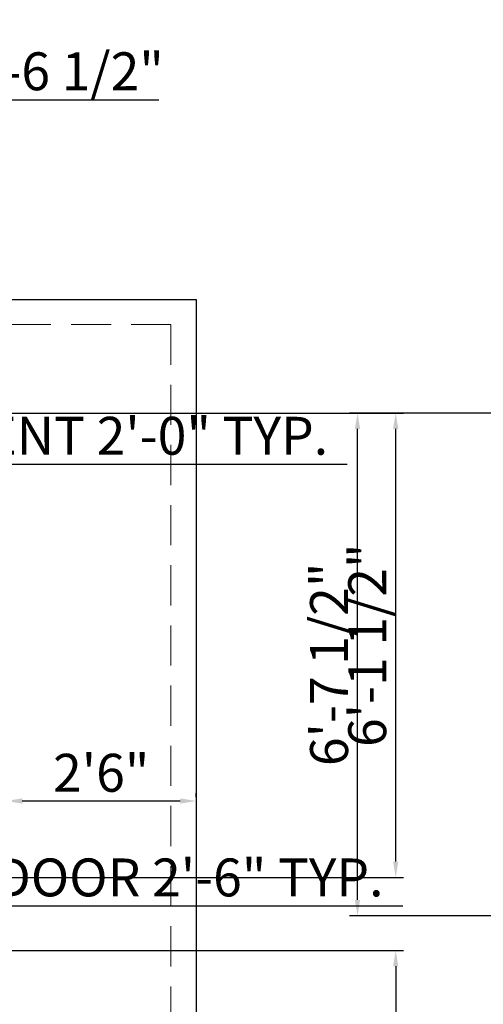
# Model space of a CAD drawing. Units: inches. Extents: x 2656 to 9931, y 1941 to 3068.
# Tile 25 of 46: x 3000 to 3074, y 2530 to 2686. Entities that reach past the tile are written whole.
import ezdxf

# ---------------------------------------------------------------- set-up
doc = ezdxf.new("R2010")
doc.units = ezdxf.units.IN
doc.linetypes.add('DASHED2', pattern=[9.525, 6.35, -3.175])
for name, color, linetype, lineweight in [('A-ANNO-DIMS', 2, 'Continuous', 18), ('A-FLOR-OVHD', 252, 'DASHED2', 13), ('C-PROP', 7, 'Continuous', 25)]:
    doc.layers.add(name, color=color, linetype=linetype, lineweight=lineweight)
doc.styles.get("Standard").update_dxf_attribs({"font": 'arial.ttf'})
doc.dimstyles.new('ISO-25', dxfattribs={"dimtxt": 6, "dimasz": 2.5, "dimexe": 1.25, "dimexo": 0.625, "dimtad": 1, "dimdec": 0, "dimlunit": 3, "dimtxsty": 'Standard', "dimcen": 2.5, "dimadec": 0, "dimazin": 0, "dimtfac": 1, "dimtdec": 0, "dimtmove": 0, "dimatfit": 3, "dimfxl": 1, "dimarcsym": 0})

# ---------------------------------------------------------------- blocks, each defined once
blk = doc.blocks.new('*D3')
at = {"layer": 'A-ANNO-DIMS', "color": 0, "lineweight": -2, "transparency": 16777216}
for p, q in [((2998.16, 2562.82), (2998.16, 2563.44)), ((3028.16, 2562.82), (3028.16, 2563.44)), ((3000.66, 2562.19), (3025.66, 2562.19))]:
    blk.add_line(p, q, dxfattribs=at)
at = {"layer": 'A-ANNO-DIMS', "color": 0, "transparency": 16777216}
for points in [[(3000.66, 2562.61), (3000.66, 2561.77), (2998.16, 2562.19)], [(3025.66, 2562.61), (3025.66, 2561.77), (3028.16, 2562.19)]]:
    blk.add_solid(points, dxfattribs=at)
at = {"layer": 'Defpoints', "color": 0, "transparency": 16777216}
for p in [(2998.16, 2562.19), (3028.16, 2562.19), (3028.16, 2562.19)]:
    blk.add_point(p, dxfattribs=at)
at = {"layer": 'A-ANNO-DIMS', "color": 0, "transparency": 16777216, "insert": (3013.16, 2565.88), "char_height": 6, "attachment_point": 5}
blk.add_mtext('2\'6"', dxfattribs=at)
blk = doc.blocks.new('*D35')
at = {"layer": 'A-ANNO-DIMS', "color": 0, "lineweight": -2, "transparency": 16777216}
for p, q in [((2946.47, 2549.48), (2946.47, 2544.33)), ((2976.57, 2549.48), (2976.57, 2544.33)), ((2948.97, 2545.58), (2974.07, 2545.58)), ((2976.57, 2545.58), (3060.91, 2545.58))]:
    blk.add_line(p, q, dxfattribs=at)
at = {"layer": 'A-ANNO-DIMS', "color": 0, "transparency": 16777216}
for points in [[(2948.97, 2546), (2948.97, 2545.17), (2946.47, 2545.58)], [(2974.07, 2546), (2974.07, 2545.17), (2976.57, 2545.58)]]:
    blk.add_solid(points, dxfattribs=at)
at = {"layer": 'Defpoints', "color": 0, "transparency": 16777216}
for p in [(2946.47, 2550.1), (2976.57, 2550.1), (2976.57, 2545.58)]:
    blk.add_point(p, dxfattribs=at)
at = {"layer": 'A-ANNO-DIMS', "color": 0, "transparency": 16777216, "insert": (3019.99, 2549.31), "char_height": 6, "attachment_point": 5}
blk.add_mtext('WC DOOR 2\'-6" TYP.', dxfattribs=at)
blk = doc.blocks.new('*D45')
at = {"layer": 'A-ANNO-DIMS', "color": 0, "lineweight": -2, "transparency": 16777216}
for p, q in [((2946.51, 2618.48), (2946.51, 2614.25)), ((2970.51, 2618.48), (2970.51, 2614.25)), ((2949.01, 2615.5), (2968.01, 2615.5)), ((2970.51, 2615.5), (3052.06, 2615.5))]:
    blk.add_line(p, q, dxfattribs=at)
at = {"layer": 'A-ANNO-DIMS', "color": 0, "transparency": 16777216}
for points in [[(2949.01, 2615.92), (2949.01, 2615.08), (2946.51, 2615.5)], [(2968.01, 2615.92), (2968.01, 2615.08), (2970.51, 2615.5)]]:
    blk.add_solid(points, dxfattribs=at)
at = {"layer": 'Defpoints', "color": 0, "transparency": 16777216}
for p in [(2946.51, 2619.1), (2970.51, 2619.1), (2970.51, 2615.5)]:
    blk.add_point(p, dxfattribs=at)
at = {"layer": 'A-ANNO-DIMS', "color": 0, "transparency": 16777216, "insert": (3012.54, 2619.23), "char_height": 6, "attachment_point": 5}
blk.add_mtext('WC VENT 2\'-0" TYP.', dxfattribs=at)
blk = doc.blocks.new('*D73')
at = {"layer": 'A-ANNO-DIMS', "color": 0, "lineweight": -2, "transparency": 16777216}
for p, q in [((3144.42, 2623.6), (3052.46, 2623.6)), ((3053.71, 2546.53), (3053.71, 2621.1)), ((3144.42, 2544.03), (3052.46, 2544.03))]:
    blk.add_line(p, q, dxfattribs=at)
at = {"layer": 'A-ANNO-DIMS', "color": 0, "transparency": 16777216}
for points in [[(3053.3, 2621.1), (3054.13, 2621.1), (3053.71, 2623.6)], [(3053.3, 2546.53), (3054.13, 2546.53), (3053.71, 2544.03)]]:
    blk.add_solid(points, dxfattribs=at)
at = {"layer": 'Defpoints', "color": 0, "transparency": 16777216}
for p in [(3053.71, 2623.6), (3145.05, 2623.6), (3145.05, 2544.03)]:
    blk.add_point(p, dxfattribs=at)
at = {"layer": 'A-ANNO-DIMS', "color": 0, "transparency": 16777216, "insert": (3049.99, 2583.82), "char_height": 6, "attachment_point": 5, "rotation": 90}
blk.add_mtext('6\'-7 1/2"', dxfattribs=at)
blk = doc.blocks.new('*D99')
at = {"layer": 'A-ANNO-DIMS', "color": 0, "lineweight": -2, "transparency": 16777216}
for p, q in [((2970.51, 2624.23), (2970.51, 2674.45)), ((2973.01, 2673.2), (2986.66, 2673.2)), ((2989.16, 2624.23), (2989.16, 2674.45)), ((2989.16, 2673.2), (3022.27, 2673.2))]:
    blk.add_line(p, q, dxfattribs=at)
at = {"layer": 'A-ANNO-DIMS', "color": 0, "transparency": 16777216}
for points in [[(2973.01, 2673.62), (2973.01, 2672.78), (2970.51, 2673.2)], [(2986.66, 2673.62), (2986.66, 2672.78), (2989.16, 2673.2)]]:
    blk.add_solid(points, dxfattribs=at)
at = {"layer": 'Defpoints', "color": 0, "transparency": 16777216}
for p in [(2989.16, 2673.2), (2970.51, 2623.6), (2989.16, 2623.6)]:
    blk.add_point(p, dxfattribs=at)
at = {"layer": 'A-ANNO-DIMS', "color": 0, "transparency": 16777216, "insert": (3006.97, 2676.93), "char_height": 6, "attachment_point": 5}
blk.add_mtext('1\'-6 1/2"', dxfattribs=at)
blk = doc.blocks.new('*D103')
at = {"layer": 'A-ANNO-DIMS', "color": 0, "lineweight": -2, "transparency": 16777216}
for p, q in [((2998.78, 2623.6), (3061.01, 2623.6)), ((3059.76, 2552.6), (3059.76, 2621.1)), ((2989.78, 2550.1), (3061.01, 2550.1))]:
    blk.add_line(p, q, dxfattribs=at)
at = {"layer": 'A-ANNO-DIMS', "color": 0, "transparency": 16777216}
for points in [[(3059.34, 2621.1), (3060.17, 2621.1), (3059.76, 2623.6)], [(3059.34, 2552.6), (3060.17, 2552.6), (3059.76, 2550.1)]]:
    blk.add_solid(points, dxfattribs=at)
at = {"layer": 'Defpoints', "color": 0, "transparency": 16777216}
for p in [(2998.16, 2623.6), (3059.76, 2623.6), (2989.16, 2550.1)]:
    blk.add_point(p, dxfattribs=at)
at = {"layer": 'A-ANNO-DIMS', "color": 0, "transparency": 16777216, "insert": (3056.03, 2586.85), "char_height": 6, "attachment_point": 5, "rotation": 90}
blk.add_mtext('6\'-1 1/2"', dxfattribs=at)
blk = doc.blocks.new('*D130')
at = {"layer": 'A-ANNO-DIMS', "color": 0, "lineweight": -2, "transparency": 16777216}
for p, q in [((2877.28, 2538.52), (3061.01, 2538.52)), ((3059.76, 2536.02), (3059.76, 2525.32)), ((2902.17, 2522.82), (3061.01, 2522.82)), ((3059.76, 2522.82), (3059.76, 2489.7))]:
    blk.add_line(p, q, dxfattribs=at)
at = {"layer": 'A-ANNO-DIMS', "color": 0, "transparency": 16777216}
for points in [[(3059.34, 2536.02), (3060.17, 2536.02), (3059.76, 2538.52)], [(3059.34, 2525.32), (3060.17, 2525.32), (3059.76, 2522.82)]]:
    blk.add_solid(points, dxfattribs=at)
at = {"layer": 'Defpoints', "color": 0, "transparency": 16777216}
for p in [(2876.66, 2538.52), (2901.54, 2522.82), (3059.76, 2522.82)]:
    blk.add_point(p, dxfattribs=at)
at = {"layer": 'A-ANNO-DIMS', "color": 0, "transparency": 16777216, "insert": (3056.03, 2505.01), "char_height": 6, "attachment_point": 5, "rotation": 90}
blk.add_mtext('1\'-3 1/2"', dxfattribs=at)

msp = doc.modelspace()

# ---------------------------------------------------------------- linework, layer by layer
at = {"layer": 'A-FLOR-OVHD'}
for p, q in [((2732.16, 2637.6), (3024.16, 2637.6)), ((3024.16, 2637.6), (3024.16, 2090.1))]:
    msp.add_line(p, q, dxfattribs=at)
at = {"layer": 'C-PROP'}
for p, q in [((2728.16, 2641.6), (3028.16, 2641.6)), ((3028.16, 2641.6), (3028.16, 2086.1))]:
    msp.add_line(p, q, dxfattribs=at)

# ---------------------------------------------------------------- dimensions: what is measured, and where the dimension line sits
at = {"layer": 'A-ANNO-DIMS'}
dim = msp.add_linear_dim(base=(2989.1573, 2673.2003), p1=(2970.5139, 2623.6003), p2=(2989.1573, 2623.6003), dimstyle='ISO-25', override={"dimdec": 1, "dimlfac": 1, "dimrnd": 0, "dimzin": 1, "dimdsep": 46, "dimlunit": 4, "dimfrac": 2}, dxfattribs=at)
dim.commit()
dim.dimension.update_dxf_attribs({"geometry": '*D99', "text_midpoint": (3006.9651, 2676.9276)})
for base, p1, p2, text, override, picture, middle in [((2970.51, 2615.5), (2946.51, 2619.1), (2970.51, 2619.1), 'WC VENT <> TYP.', {"dimdec": 1, "dimlfac": 1, "dimrnd": 0, "dimzin": 1, "dimdsep": 46, "dimlunit": 4, "dimfrac": 2}, '*D45', (3012.54, 2619.23)), ((3028.16, 2562.19), (2998.16, 2562.19), (3028.16, 2562.19), '2\'6"', {"dimclrd": 0, "dimclre": 0, "dimclrt": 0}, '*D3', (3013.16, 2565.88)), ((2976.57, 2545.58), (2946.47, 2550.1), (2976.57, 2550.1), 'WC DOOR <> TYP.', {"dimdec": 1, "dimlfac": 1, "dimrnd": 0, "dimzin": 1, "dimdsep": 46, "dimlunit": 4, "dimfrac": 2}, '*D35', (3019.99, 2549.31))]:
    dim = msp.add_linear_dim(base=base, p1=p1, p2=p2, text=text, dimstyle='ISO-25', override=override, dxfattribs=at)
    dim.commit()
    dim.dimension.update_dxf_attribs({"geometry": picture, "text_midpoint": middle})
for base, p1, p2, picture, middle in [((3059.76, 2623.6), (2989.16, 2550.1), (2998.16, 2623.6), '*D103', (3056.03, 2586.85)), ((3053.71, 2623.6), (3145.05, 2544.03), (3145.05, 2623.6), '*D73', (3049.99, 2583.82)), ((3059.76, 2522.82), (2876.66, 2538.52), (2901.54, 2522.82), '*D130', (3056.03, 2505.01))]:
    dim = msp.add_linear_dim(base=base, p1=p1, p2=p2, angle=90, dimstyle='ISO-25', override={"dimdec": 1, "dimlfac": 1, "dimrnd": 0, "dimzin": 1, "dimdsep": 46, "dimlunit": 4, "dimfrac": 2}, dxfattribs=at)
    dim.commit()
    dim.dimension.update_dxf_attribs({"geometry": picture, "text_midpoint": middle})

doc.saveas('drawing.dxf')
